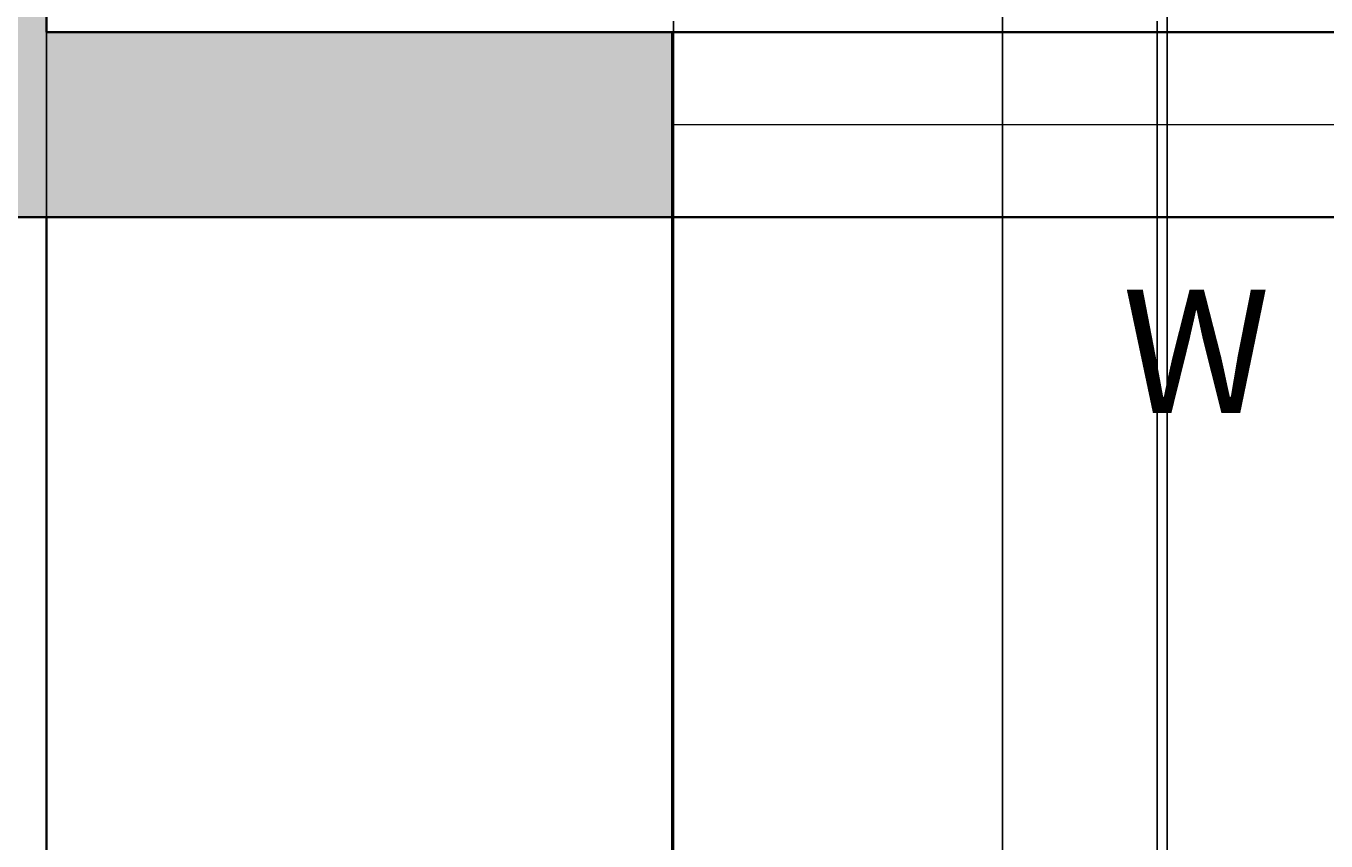
# Model space of a CAD drawing. Units: inches. Extents: x -5 to 330, y -522 to 40.
# Tile 4 of 23: x 32 to 95, y -457 to -417. Entities that reach past the tile are written whole.
import ezdxf

# ---------------------------------------------------------------- set-up
doc = ezdxf.new("R2010")
doc.units = ezdxf.units.IN
doc.header["$MEASUREMENT"] = 0
for name, color, linetype, lineweight in [('A-ANNO-DIMS', 2, 'Continuous', 18), ('A-ANNO-TEXT', 7, 'Continuous', 18), ('A-GLAZ', 4, 'Continuous', 18), ('A-SITE-WALL', 7, 'Continuous', 35), ('A-WALL', 7, 'Continuous', 35)]:
    doc.layers.add(name, color=color, linetype=linetype, lineweight=lineweight)
doc.layers.add('A-WALL-PATT', color=18, linetype='Continuous', lineweight=13, true_color=0x000000)
doc.styles.get("Standard").update_dxf_attribs({"font": 'arial.ttf'})
doc.dimstyles.get("Standard").update_dxf_attribs({"dimtxt": 0.18, "dimasz": 0.18, "dimexe": 0.18, "dimexo": 0.0625, "dimgap": 0.09, "dimtad": 0, "dimtih": 1, "dimtoh": 1, "dimdec": 0, "dimzin": 0, "dimdsep": 46, "dimlunit": 3, "dimtxsty": 'Standard', "dimcen": 0.09, "dimadec": 0, "dimazin": 0, "dimtfac": 1, "dimtdec": 0, "dimtofl": 0, "dimtmove": 0, "dimatfit": 3, "dimfxl": 1, "dimtolj": 1, "dimtzin": 0, "dimarcsym": 0})

# ---------------------------------------------------------------- blocks, each defined once
blk = doc.blocks.new('WIN-60IN-GLAZ')
for p, q in [((0, 9), (60, 9)), ((0, 4.5), (60, 4.5)), ((60, 0), (0, 0))]:
    blk.add_line(p, q)
blk = doc.blocks.new('*D40')
at = {"layer": 'A-ANNO-DIMS', "color": 0, "lineweight": -2, "transparency": 16777216}
for p, q in [((32.51, -246.706), (32.51, -522.309)), ((79.01, -246.706), (79.01, -522.309)), ((32.69, -522.129), (55.151, -522.129)), ((78.83, -522.129), (56.369, -522.129))]:
    blk.add_line(p, q, dxfattribs=at)
at = {"layer": 'A-ANNO-DIMS', "color": 0, "transparency": 16777216}
for points in [[(32.69, -522.099), (32.69, -522.159), (32.51, -522.129)], [(78.83, -522.099), (78.83, -522.159), (79.01, -522.129)]]:
    blk.add_solid(points, dxfattribs=at)
at = {"layer": 'Defpoints', "color": 0, "transparency": 16777216}
for p in [(32.51, -246.644), (79.01, -246.644), (79.01, -522.129)]:
    blk.add_point(p, dxfattribs=at)
at = {"layer": 'A-ANNO-DIMS', "color": 0, "transparency": 16777216, "insert": (55.76, -522.129), "char_height": 0.18, "attachment_point": 5}
blk.add_mtext('\\A1;3\'-10 1/2"', dxfattribs=at)
blk = doc.blocks.new('*D41')
at = {"layer": 'A-ANNO-DIMS', "color": 0, "lineweight": -2, "transparency": 16777216}
for p, q in [((87.01, -246.706), (87.01, -522.309)), ((129.01, -246.706), (129.01, -522.309)), ((87.19, -522.129), (107.681, -522.129)), ((128.83, -522.129), (108.339, -522.129))]:
    blk.add_line(p, q, dxfattribs=at)
at = {"layer": 'A-ANNO-DIMS', "color": 0, "transparency": 16777216}
for points in [[(87.19, -522.099), (87.19, -522.159), (87.01, -522.129)], [(128.83, -522.099), (128.83, -522.159), (129.01, -522.129)]]:
    blk.add_solid(points, dxfattribs=at)
at = {"layer": 'Defpoints', "color": 0, "transparency": 16777216}
for p in [(87.01, -246.644), (129.01, -246.644), (129.01, -522.129)]:
    blk.add_point(p, dxfattribs=at)
at = {"layer": 'A-ANNO-DIMS', "color": 0, "transparency": 16777216, "insert": (108.01, -522.129), "char_height": 0.18, "attachment_point": 5}
blk.add_mtext('\\A1;3\'-6"', dxfattribs=at)
blk = doc.blocks.new('*D45')
at = {"layer": 'A-ANNO-DIMS', "color": 0, "lineweight": -2, "transparency": 16777216}
for p, q in [((32.51, -417.206), (32.51, -522.309)), ((62.918, -417.206), (62.918, -522.309)), ((32.69, -522.129), (47.173, -522.129)), ((62.738, -522.129), (48.254, -522.129))]:
    blk.add_line(p, q, dxfattribs=at)
at = {"layer": 'A-ANNO-DIMS', "color": 0, "transparency": 16777216}
for points in [[(32.69, -522.099), (32.69, -522.159), (32.51, -522.129)], [(62.738, -522.099), (62.738, -522.159), (62.918, -522.129)]]:
    blk.add_solid(points, dxfattribs=at)
at = {"layer": 'Defpoints', "color": 0, "transparency": 16777216}
for p in [(32.51, -417.144), (62.918, -417.144), (62.918, -522.129)]:
    blk.add_point(p, dxfattribs=at)
at = {"layer": 'A-ANNO-DIMS', "color": 0, "transparency": 16777216, "insert": (47.714, -522.129), "char_height": 0.18, "attachment_point": 5}
blk.add_mtext('\\A1;2\'-6 1/2"', dxfattribs=at)
blk = doc.blocks.new('*D48')
at = {"layer": 'A-ANNO-DIMS', "color": 0, "lineweight": -2, "transparency": 16777216}
for p, q in [((63.01, -416.607), (63.01, -522.309)), ((86.523, -416.607), (86.523, -522.309)), ((63.19, -522.129), (74.166, -522.129)), ((86.343, -522.129), (75.367, -522.129))]:
    blk.add_line(p, q, dxfattribs=at)
at = {"layer": 'A-ANNO-DIMS', "color": 0, "transparency": 16777216}
for points in [[(63.19, -522.099), (63.19, -522.159), (63.01, -522.129)], [(86.343, -522.099), (86.343, -522.159), (86.523, -522.129)]]:
    blk.add_solid(points, dxfattribs=at)
at = {"layer": 'Defpoints', "color": 0, "transparency": 16777216}
for p in [(63.01, -416.544), (86.523, -416.544), (86.523, -522.129)]:
    blk.add_point(p, dxfattribs=at)
at = {"layer": 'A-ANNO-DIMS', "color": 0, "transparency": 16777216, "insert": (74.767, -522.129), "char_height": 0.18, "attachment_point": 5}
blk.add_mtext('\\A1;1\'-11 1/2"', dxfattribs=at)
blk = doc.blocks.new('*D50')
at = {"layer": 'A-ANNO-DIMS', "color": 0, "lineweight": -2, "transparency": 16777216}
for p, q in [((32.51, -417.206), (32.51, -522.309)), ((23.51, -426.206), (23.51, -522.309)), ((23.69, -522.129), (27.681, -522.129)), ((32.33, -522.129), (28.339, -522.129))]:
    blk.add_line(p, q, dxfattribs=at)
at = {"layer": 'A-ANNO-DIMS', "color": 0, "transparency": 16777216}
for points in [[(23.69, -522.099), (23.69, -522.159), (23.51, -522.129)], [(32.33, -522.099), (32.33, -522.159), (32.51, -522.129)]]:
    blk.add_solid(points, dxfattribs=at)
at = {"layer": 'Defpoints', "color": 0, "transparency": 16777216}
for p in [(32.51, -417.144), (23.51, -426.144), (32.51, -522.129)]:
    blk.add_point(p, dxfattribs=at)
at = {"layer": 'A-ANNO-DIMS', "color": 0, "transparency": 16777216, "insert": (28.01, -522.129), "char_height": 0.18, "attachment_point": 5}
blk.add_mtext('\\A1;0\'-9"', dxfattribs=at)

msp = doc.modelspace()

# ---------------------------------------------------------------- hatches: boundary and pattern name
at = {"layer": 'A-WALL-PATT'}
h = msp.add_hatch(color=256, dxfattribs=at)
h.dxf.hatch_style = 1
h.paths.add_polyline_path([(164.01, -44.152), (159.51, -44.152), (159.51, -153.144), (164.01, -153.144)], flags=17)
h.paths.add_polyline_path([(224.01, -188.144), (272.01, -188.144), (272.01, -218.144), (260.01, -218.144), (260.01, -222.644), (272.01, -222.644), (272.01, -292.644), (159.01, -292.644), (159.01, -297.144), (272.01, -297.144), (272.01, -417.144), (245.51, -417.144), (245.51, -426.144), (272.01, -426.144), (272.01, -495.144), (281.01, -495.144), (281.01, 12.356), (23.51, 12.356), (23.51, -426.144), (62.918, -426.144), (62.918, -417.144), (32.51, -417.144), (32.51, -297.144), (48.129, -297.144), (48.129, -292.644), (32.51, -292.644), (32.51, -140.644), (133.51, -140.644), (133.51, -131.644), (32.51, -131.644), (32.51, 3.356), (159.51, 3.356), (164.01, 3.356), (220.01, 3.356), (224.51, 3.356), (272.01, 3.356), (272.01, -179.144), (159.51, -179.144), (159.51, -188.144), (219.51, -188.144), (219.51, -266.644), (224.01, -266.644), (224.01, -222.644), (236.01, -222.644), (236.01, -218.144), (224.01, -218.144)])
h.paths.add_polyline_path([(133.01, -292.644), (128.51, -292.644), (128.51, -297.144), (128.51, -417.144), (122.918, -417.144), (122.918, -426.144), (133.01, -426.144)], flags=17)
h.paths.add_polyline_path([(185.51, -417.144), (159.01, -417.144), (159.01, -426.144), (185.51, -426.144)], flags=17)
h.paths.add_polyline_path([(133.51, -140.644), (129.01, -140.644), (129.01, -246.644), (133.51, -246.644)], flags=17)
h.paths.add_polyline_path([(246.01, -48.644), (224.51, -48.644), (224.51, -27.627), (220.01, -27.627), (220.01, -48.644), (198.604, -48.644), (198.604, -53.144), (246.01, -53.144)], flags=17)

# ---------------------------------------------------------------- linework, layer by layer
at = {"layer": 'A-GLAZ'}
msp.add_line((62.918, -426.144), (62.918, -417.144), dxfattribs=at)
at = {"layer": 'A-SITE-WALL'}
msp.add_line((32.51, -426.144), (32.51, -495.144), dxfattribs=at)
at = {"layer": 'A-WALL'}
for p, q in [((32.51, -297.144), (32.51, -417.144)), ((32.51, -417.144), (128.51, -417.144)), ((23.51, -426.144), (135.01, -426.144))]:
    msp.add_line(p, q, dxfattribs=at)

# ---------------------------------------------------------------- block references
at = {"layer": 'A-GLAZ'}
msp.add_blockref('WIN-60IN-GLAZ', (62.918, -426.144), dxfattribs=at)

# ---------------------------------------------------------------- texts
at = {"layer": 'A-ANNO-TEXT', "insert": (84.84, -429.673), "char_height": 6, "attachment_point": 1}
msp.add_mtext('W', dxfattribs=at)

# ---------------------------------------------------------------- dimensions: what is measured, and where the dimension line sits
at = {"layer": 'A-ANNO-DIMS'}
for base, p1, p2, picture, middle in [((79.01, -522.129), (32.51, -246.644), (79.01, -246.644), '*D40', (55.76, -522.129)), ((129.01, -522.129), (87.01, -246.644), (129.01, -246.644), '*D41', (108.01, -522.129)), ((86.523, -522.129), (63.01, -416.544), (86.523, -416.544), '*D48', (74.767, -522.129)), ((32.51, -522.129), (23.51, -426.144), (32.51, -417.144), '*D50', (28.01, -522.129)), ((62.918, -522.129), (32.51, -417.144), (62.918, -417.144), '*D45', (47.714, -522.129))]:
    dim = msp.add_linear_dim(base=base, p1=p1, p2=p2, dimstyle='Standard', override={"dimdec": 1, "dimlfac": 1, "dimrnd": 0, "dimzin": 1, "dimdsep": 46, "dimlunit": 4, "dimfrac": 2}, dxfattribs=at)
    dim.commit()
    dim.dimension.update_dxf_attribs({"geometry": picture, "text_midpoint": middle})

doc.saveas('drawing.dxf')
